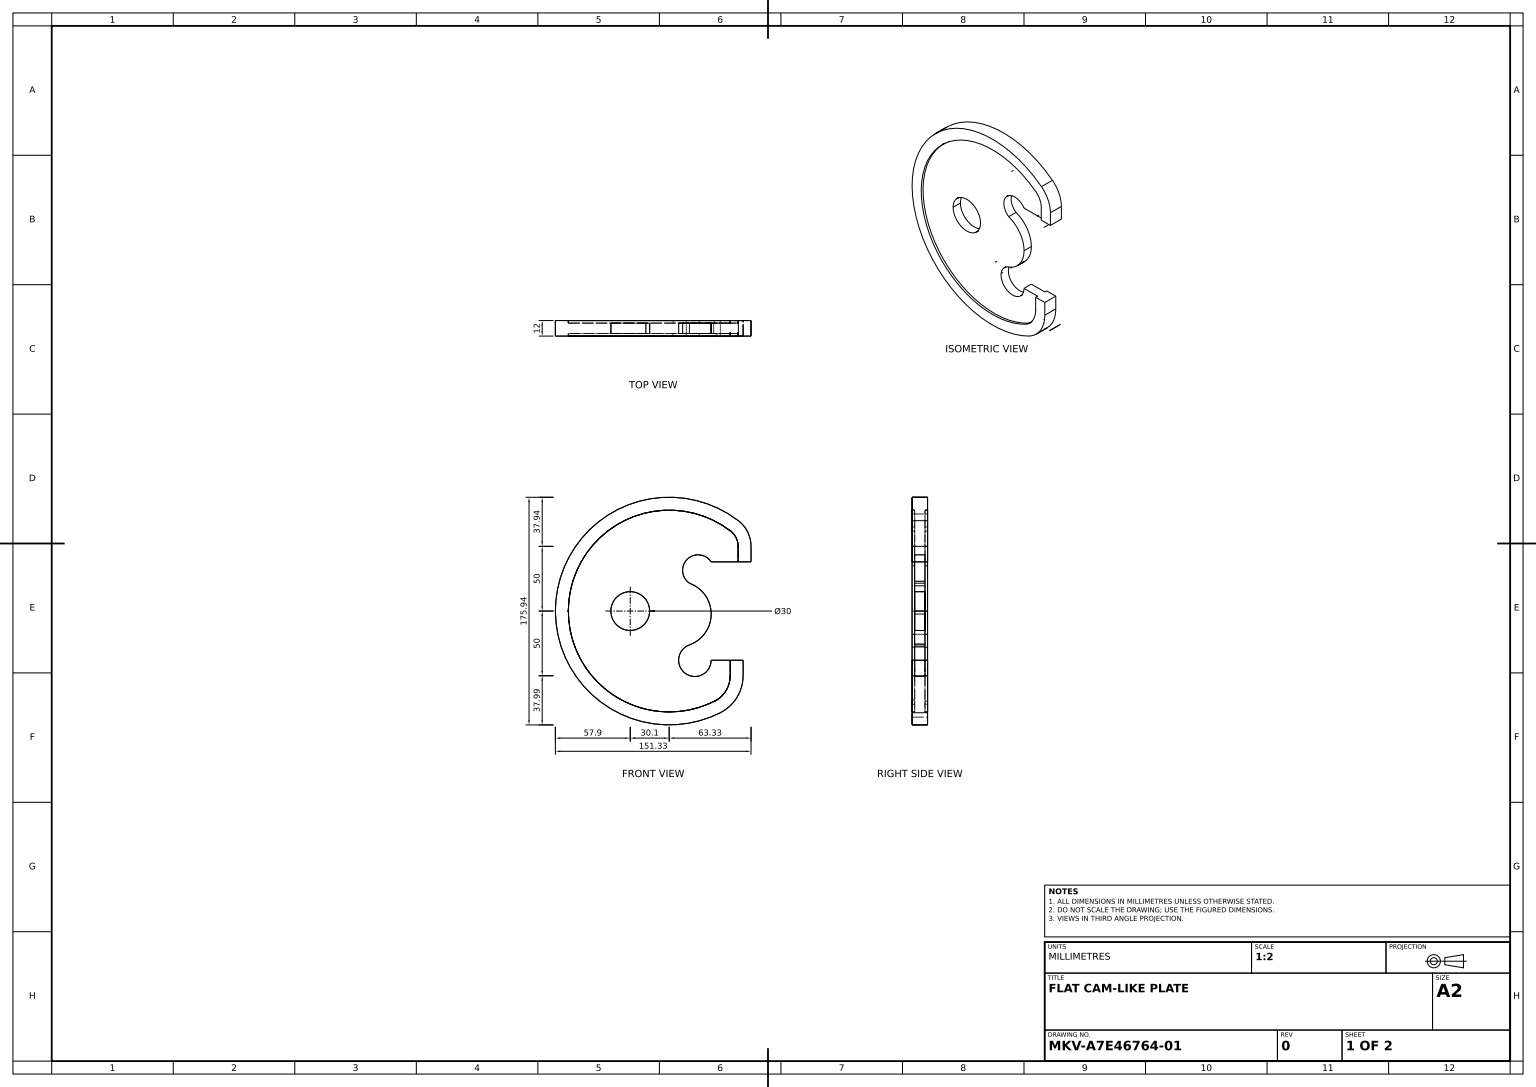
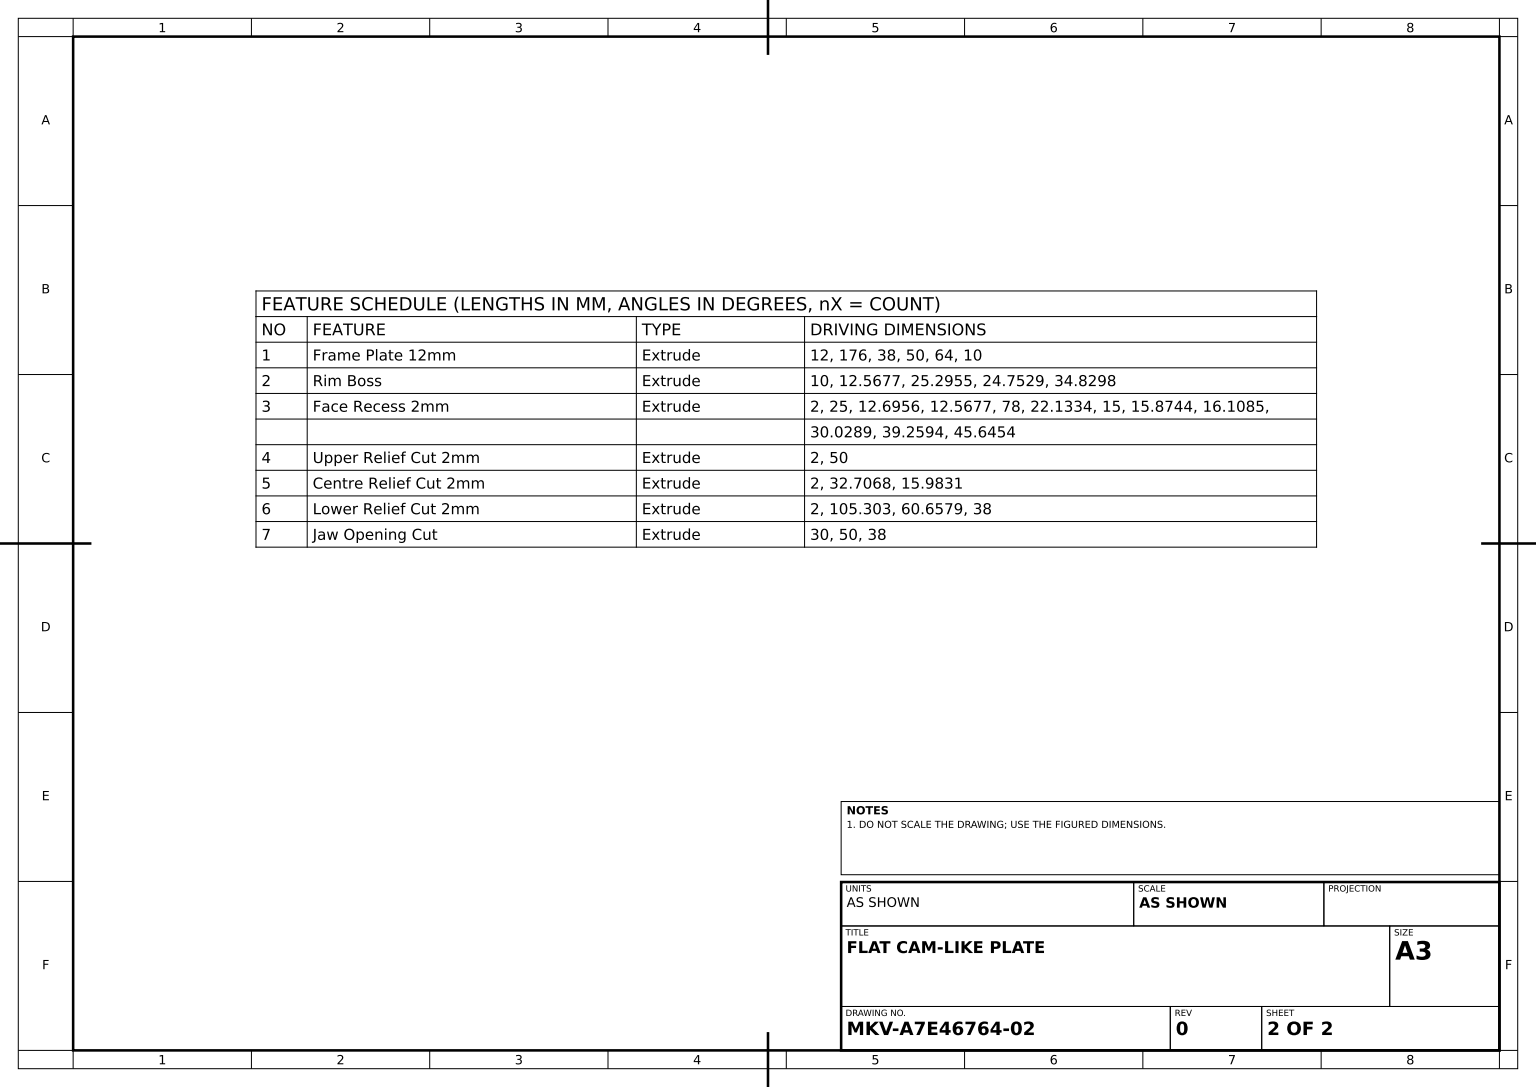
SolidWorks part; units mm, degrees
material "Plain Carbon Steel"
ref_plane "Front Plane" through (0, 0, 0) normal (0, 0, 1) x (1, 0, 0)
ref_plane "Top Plane" through (0, 0, 0) normal (0, 1, 0) x (1, 0, 0)
ref_plane "Right Plane" through (0, 0, 0) normal (1, 0, 0) x (0, 0, -1)
sketch "Frame Profile Sketch" plane through (0, 0, 0) normal (0, 0, 1) x (1, 0, 0)
  line L0 (0, 0) -> (88, 0) construction
  line L1 (88, 0) -> (88, 38) construction
  line L2 (88, -38) -> (0, -38) construction
  line L3 (88, 38) -> (0, 38) construction
  line L4 (88, -50) -> (88, 50) construction
  line L5 (88, 50) -> (-9.0689, 50) construction
  line L6 (88, -50) -> (-9.0689, -50) construction
  line L7 (57.219, -50) -> (57.219, -38)
  line L8 (63.3275, 50) -> (63.3275, 38)
  line L9 (53.3275, 50) -> (53.3275, 38)
  line L10 (47.219, -50) -> (47.219, -38)
  line L11 (53.3275, 38) -> (63.3275, 38)
  line L12 (47.219, -38) -> (57.219, -38)
  arc A0 (53.5369, 69.8413) -> (39.6299, -78.5714) centre (0, 0) ccw
  arc A10 (63.3275, 50) -> (53.5369, 69.8413) centre (38.3275, 50) ccw
  arc A11 (39.6299, -78.5714) -> (57.219, -50) centre (25.219, -50) ccw
  arc A12 (53.3275, 50) -> (47.4531, 61.9048) centre (38.3275, 50) ccw
  arc A13 (47.4531, 61.9048) -> (35.1265, -69.6429) centre (0, 0) ccw
  arc A14 (35.1265, -69.6429) -> (47.219, -50) centre (25.219, -50) ccw
  dimension "D1" = 176
  dimension "D4" = 50
  dimension "D3" = 50
  dimension "D5" = 64
  dimension "D2" = 38
  dimension "D6" = 10
extrude "Frame Plate 12mm" add sketch "Frame Profile Sketch" along normal mid plane 12
sketch "Rim Boss Sketch" plane through (0, 0, 6) normal (0, 0, 1) x (1, 0, 0)
  line L0 (53.3275, 38) -> (32.4662, 38)
  line L1 (47.219, -38) -> (32.4662, -38)
  line L2 (57.219, -50) -> (57.219, -38) construction
  line L8 (57.219, -50) -> (57.219, -38)
  line L9 (57.219, -38) -> (47.219, -38)
  line L10 (47.219, -38) -> (47.219, -50)
  line L11 (53.3275, 50) -> (53.3275, 38)
  line L12 (53.3275, 38) -> (63.3275, 38)
  line L13 (63.3275, 38) -> (63.3275, 50)
  line L16 (47.219, -38) -> (47.219, -50)
  line L17 (53.3275, 50) -> (53.3275, 38)
  arc A0 (32.4662, 38) -> (15.6965, 21.5239) centre (22.3892, 31.4842) ccw
  arc A1 (32.4662, -38) -> (15.6965, -26.1556) centre (19.8985, -38) cw
  arc A2 (15.6965, -26.1556) -> (15.6965, 21.5239) centre (7.2391, -2.3158) ccw
  arc A9 (39.6299, -78.5714) -> (57.219, -50) centre (25.219, -50) ccw
  arc A10 (35.1265, -69.6429) -> (47.219, -50) centre (25.219, -50) ccw
  arc A11 (47.4531, 61.9048) -> (35.1265, -69.6429) centre (0, 0) ccw
  arc A12 (53.3275, 50) -> (47.4531, 61.9048) centre (38.3275, 50) ccw
  arc A13 (63.3275, 50) -> (53.5369, 69.8413) centre (38.3275, 50) ccw
  arc A14 (53.5369, 69.8413) -> (39.6299, -78.5714) centre (0, 0) ccw
  arc A16 (35.1265, -69.6429) -> (47.219, -50) centre (25.219, -50) ccw
  arc A17 (47.4531, 61.9048) -> (35.1265, -69.6429) centre (0, 0) ccw
  arc A18 (53.3275, 50) -> (47.4531, 61.9048) centre (38.3275, 50) ccw
  dimension "D1" = 0
  dimension "D2" = 12.5677
  dimension "D3" = 25.2955
  dimension "D4" = 24.7529
  dimension "D5" = 34.8298
extrude "Rim Boss" add sketch "Rim Boss Sketch" against normal blind 10
sketch "Face Recess Sketch" plane through (0, 0, 6) normal (0, 0, 1) x (1, 0, 0)
  line L0 (47.219, -50) -> (47.219, -38)
  line L1 (57.219, -38) -> (32.4662, -38) construction
  line L2 (47.219, -38) -> (32.4662, -38)
  line L3 (53.3275, 50) -> (53.3275, 38)
  line L4 (53.3275, 38) -> (32.4662, 38)
  line L5 (63.3275, 38) -> (63.3275, 50) construction
  arc A1 (32.4662, 38) -> (17.6821, 20.446) centre (22.3892, 31.4842) ccw
  arc A2 (15.644, -25.9029) -> (17.6821, 20.446) centre (7.3497, -2.3189) ccw
  arc A4 (24.0681, -49.8558) -> (15.644, -25.9029) centre (19.8561, -37.8794) cw
  arc A5 (32.4662, -38) -> (24.0681, -49.8558) centre (19.8985, -38) cw
  arc A6 (47.4531, 61.9048) -> (36.8667, -68.7375) centre (0, 0) ccw
  arc A7 (47.219, -50) -> (33.2986, -70.5532) centre (25.0856, -50) cw
  arc A11 (53.3275, 50) -> (47.4531, 61.9048) centre (38.3275, 50) ccw
  arc M6 (15.6965, 21.5239) -> (32.4662, 38) centre (22.3892, 31.4842) cw
  line M7 (32.4662, 38) -> (63.3275, 38)
  line M13 (57.219, -38) -> (32.4662, -38)
  arc M14 (32.4662, -38) -> (15.6965, -26.1556) centre (19.8985, -38) cw
  dimension "D1" = 25
  dimension "D2" = 12.6956
  dimension "D3" = 12.5677
  dimension "D4" = 78
  dimension "D5" = 22.1334
  dimension "D6" = 15
  dimension "D7" = 15.8744
  dimension "D8" = 16.1085
  dimension "D9" = 30.0289
  dimension "D10" = 39.2594
  dimension "D11" = 45.6454
extrude "Face Recess 2mm" cut sketch "Face Recess Sketch" against normal blind 2 contours L3 A11 A6 A7 L0 A4 A2 A1 M13 M14 M6 M7
sketch "Upper Relief Cut Sketch" plane through (0, 0, 4) normal (0, 0, 1) x (1, 0, 0)
  circle A0 centre (7.3497, -2.3189) radius 25
  dimension "D1" = 50
extrude "Upper Relief Cut 2mm" cut sketch "Upper Relief Cut Sketch" along normal blind 2
sketch "Centre Relief Cut Sketch" plane through (0, 0, 4) normal (0, 0, 1) x (1, 0, 0)
  arc A0 (23.8332, -22.399) -> (4.8623, -32.3434) centre (0, 0) ccw
  arc A1 (4.8623, -32.3434) -> (23.8332, -22.399) centre (19.8561, -37.8794) ccw
  dimension "D1" = 32.7068
  dimension "D2" = 15.9831
extrude "Centre Relief Cut 2mm" cut sketch "Centre Relief Cut Sketch" along normal blind 2
sketch "Lower Relief Cut Sketch" plane through (0, 0, 4) normal (0, 0, 1) x (1, 0, 0)
  line L0 (53.3275, 50) -> (53.3275, 38) construction
  line L1 (32.4662, 38) -> (53.3275, 38) construction
  circle A0 centre (-7.3304, 0) radius 52.6515
  dimension "D1" = 105.303
  dimension "D2" = 60.6579
  dimension "D3" = 38
extrude "Lower Relief Cut 2mm" cut sketch "Lower Relief Cut Sketch" along normal blind 2
sketch "Jaw Opening Sketch" plane through (0, 0, 4) normal (0, 0, 1) x (1, 0, 0)
  line L0 (19.8985, -38) -> (-30.1015, -38) construction
  line L1 (-30.1015, -38) -> (-30.1015, 0) construction
  line L3 (32.4662, 38) -> (53.3275, 38) construction
  circle A0 centre (-30.1015, 0) radius 15
  dimension "D1" = 30
  dimension "D2" = 50
  dimension "D3" = 38
extrude "Jaw Opening Cut" cut sketch "Jaw Opening Sketch" against normal through all
